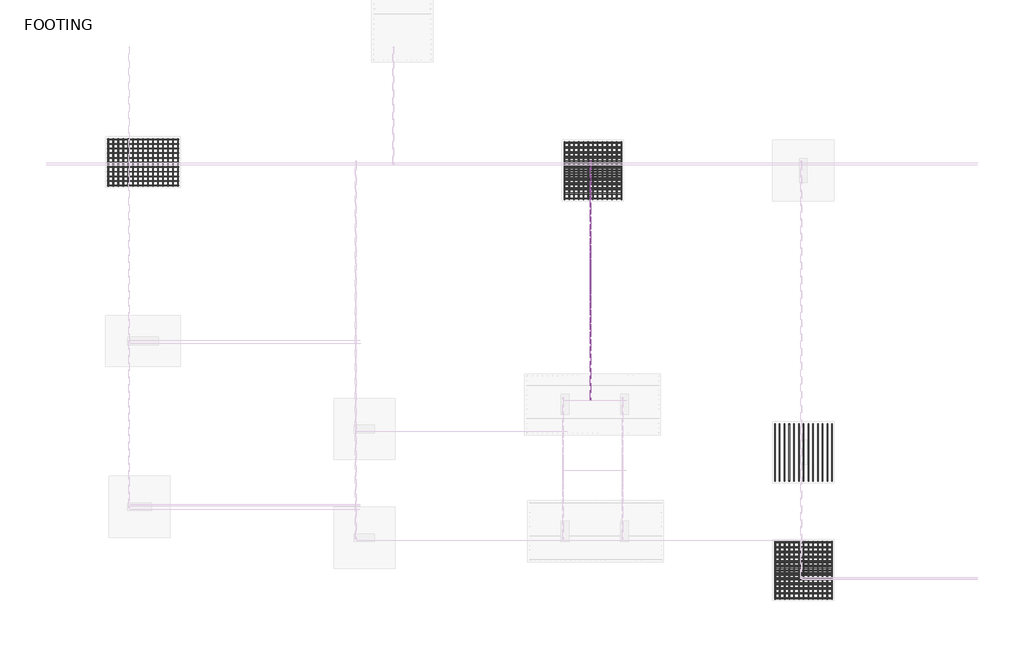
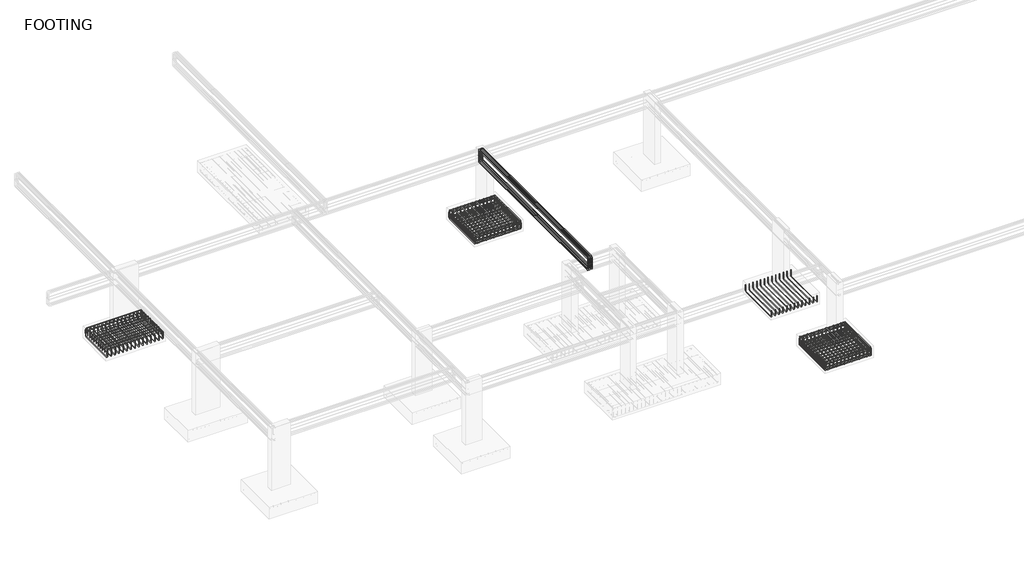
# One storey, part 5 of 12: 15 reinforcing bars.
"""IFC4 building model written with IfcOpenShell, lengths in millimetres."""

from ifc_helpers import new_model, si_unit, point, frame, origin, place, context, project, spatial, polyline, circle_curve, trimmed, segment, composite_curve, source, transform, mapped, element, save
from ifc_brep_helpers import swept_disk

model = new_model("IFC4")

# Units and contexts
model_context = context("Model", 3, world=origin())
ifc_project = project(units=[si_unit("LENGTHUNIT", "METRE", prefix="MILLI")], contexts=[model_context])

# Site, building, storey
site = spatial("IfcSite", under=ifc_project)
building = spatial("IfcBuilding", under=site)
storey = spatial("IfcBuildingStorey", under=building, Name="FOOTING", Elevation=-5638.8)

# Reinforcing bars
placement = place(None, origin())
reinforcing_bar_shape = source(origin(), model_context, "Body", "SolidModel", [
    swept_disk(composite_curve([segment(polyline([(5332.7998335, -15010.4541655, -5788.8), (5332.7998335, -15010.4541655, -5975.4)]), True, "CONTINUOUS"), segment(trimmed(circle_curve(frame((5332.7998335, -14955.0041655, -5975.4), z_axis=(1.0, 0.0, 0.0), x_axis=(0.0, -55.44999999999891, 0.0)), 55.45), [point((5332.7998335, -15010.4541655, -5975.4))], [point((5332.7998335, -14955.0041655, -6030.85))], True, "CARTESIAN"), True, "CONTINUOUS"), segment(polyline([(5332.7998335, -14955.0041655, -6030.85), (5332.7998335, -13381.8041655, -6030.85)]), True, "CONTINUOUS"), segment(trimmed(circle_curve(frame((5332.7998335, -13381.8041655, -5975.4), z_axis=(1.0, 0.0, 0.0), x_axis=(0.0, 0.0, -55.45000000000073)), 55.45), [point((5332.7998335, -13381.8041655, -6030.85))], [point((5332.7998335, -13326.3541655, -5975.4))], True, "CARTESIAN"), True, "CONTINUOUS"), segment(polyline([(5332.7998335, -13326.3541655, -5975.4), (5332.7998335, -13326.3541655, -5788.8)]), True, "CONTINUOUS")], self_intersect=False), 7.95),
])
element("IfcReinforcingBar", 1, at=placement, inside=storey, context=model_context, shape_type="MappedRepresentation", body=[
    mapped(reinforcing_bar_shape, transform((0.0, 0.0, 0.0), x_axis=(1.0, 0.0, 0.0), y_axis=(0.0, 1.0, 0.0), z_axis=(0.0, 0.0, 1.0))),
    mapped(reinforcing_bar_shape, transform((-140.3416667, 0.0, 0.0), x_axis=(1.0, 0.0, 0.0), y_axis=(0.0, 1.0, 0.0), z_axis=(0.0, 0.0, 1.0))),
    mapped(reinforcing_bar_shape, transform((-280.6833333, 0.0, 0.0), x_axis=(1.0, 0.0, 0.0), y_axis=(0.0, 1.0, 0.0), z_axis=(0.0, 0.0, 1.0))),
    mapped(reinforcing_bar_shape, transform((-421.025, 0.0, 0.0), x_axis=(1.0, 0.0, 0.0), y_axis=(0.0, 1.0, 0.0), z_axis=(0.0, 0.0, 1.0))),
    mapped(reinforcing_bar_shape, transform((-561.3666667, 0.0, 0.0), x_axis=(1.0, 0.0, 0.0), y_axis=(0.0, 1.0, 0.0), z_axis=(0.0, 0.0, 1.0))),
    mapped(reinforcing_bar_shape, transform((-701.7083333, 0.0, 0.0), x_axis=(1.0, 0.0, 0.0), y_axis=(0.0, 1.0, 0.0), z_axis=(0.0, 0.0, 1.0))),
    mapped(reinforcing_bar_shape, transform((-842.05, 0.0, 0.0), x_axis=(1.0, 0.0, 0.0), y_axis=(0.0, 1.0, 0.0), z_axis=(0.0, 0.0, 1.0))),
    mapped(reinforcing_bar_shape, transform((-982.3916667, 0.0, 0.0), x_axis=(1.0, 0.0, 0.0), y_axis=(0.0, 1.0, 0.0), z_axis=(0.0, 0.0, 1.0))),
    mapped(reinforcing_bar_shape, transform((-1122.7333333, 0.0, 0.0), x_axis=(1.0, 0.0, 0.0), y_axis=(0.0, 1.0, 0.0), z_axis=(0.0, 0.0, 1.0))),
    mapped(reinforcing_bar_shape, transform((-1263.075, 0.0, 0.0), x_axis=(1.0, 0.0, 0.0), y_axis=(0.0, 1.0, 0.0), z_axis=(0.0, 0.0, 1.0))),
    mapped(reinforcing_bar_shape, transform((-1403.4166667, 0.0, 0.0), x_axis=(1.0, 0.0, 0.0), y_axis=(0.0, 1.0, 0.0), z_axis=(0.0, 0.0, 1.0))),
    mapped(reinforcing_bar_shape, transform((-1543.7583333, 0.0, 0.0), x_axis=(1.0, 0.0, 0.0), y_axis=(0.0, 1.0, 0.0), z_axis=(0.0, 0.0, 1.0))),
    mapped(reinforcing_bar_shape, transform((-1684.1, 0.0, 0.0), x_axis=(1.0, 0.0, 0.0), y_axis=(0.0, 1.0, 0.0), z_axis=(0.0, 0.0, 1.0))),
])
reinforcing_bar_2_shape = source(origin(), model_context, "Body", "SolidModel", [
    swept_disk(composite_curve([segment(polyline([(5323.6597994, -13324.7541655, -5888.8), (5323.6597994, -13324.7541655, -5741.5)]), True, "CONTINUOUS"), segment(trimmed(circle_curve(frame((5323.6597994, -13371.1041655, -5741.5), z_axis=(1.0, 0.0, 0.0), x_axis=(0.0, 46.350000000000364, 0.0)), 46.35), [point((5323.6597994, -13324.7541655, -5741.5))], [point((5323.6597994, -13371.1041655, -5695.15))], True, "CARTESIAN"), True, "CONTINUOUS"), segment(polyline([(5323.6597994, -13371.1041655, -5695.15), (5323.6597994, -14965.7041655, -5695.15)]), True, "CONTINUOUS"), segment(trimmed(circle_curve(frame((5323.6597994, -14965.7041655, -5741.5), z_axis=(1.0, 0.0, 0.0), x_axis=(0.0, 0.0, 46.350000000000364)), 46.35), [point((5323.6597994, -14965.7041655, -5695.15))], [point((5323.6597994, -15012.0541655, -5741.5))], True, "CARTESIAN"), True, "CONTINUOUS"), segment(polyline([(5323.6597994, -15012.0541655, -5741.5), (5323.6597994, -15012.0541655, -5888.8)]), True, "CONTINUOUS")], self_intersect=False), 6.35),
])
element("IfcReinforcingBar", 2, at=placement, inside=storey, context=model_context, shape_type="MappedRepresentation", body=[
    mapped(reinforcing_bar_2_shape, transform((0.0, 0.0, 0.0), x_axis=(1.0, 0.0, 0.0), y_axis=(0.0, 1.0, 0.0), z_axis=(0.0, 0.0, 1.0))),
    mapped(reinforcing_bar_2_shape, transform((-138.4829293, 0.0, 0.0), x_axis=(1.0, 0.0, 0.0), y_axis=(0.0, 1.0, 0.0), z_axis=(0.0, 0.0, 1.0))),
    mapped(reinforcing_bar_2_shape, transform((-276.9658586, 0.0, 0.0), x_axis=(1.0, 0.0, 0.0), y_axis=(0.0, 1.0, 0.0), z_axis=(0.0, 0.0, 1.0))),
    mapped(reinforcing_bar_2_shape, transform((-415.4487879, 0.0, 0.0), x_axis=(1.0, 0.0, 0.0), y_axis=(0.0, 1.0, 0.0), z_axis=(0.0, 0.0, 1.0))),
    mapped(reinforcing_bar_2_shape, transform((-553.9317172, 0.0, 0.0), x_axis=(1.0, 0.0, 0.0), y_axis=(0.0, 1.0, 0.0), z_axis=(0.0, 0.0, 1.0))),
    mapped(reinforcing_bar_2_shape, transform((-692.4146465, 0.0, 0.0), x_axis=(1.0, 0.0, 0.0), y_axis=(0.0, 1.0, 0.0), z_axis=(0.0, 0.0, 1.0))),
    mapped(reinforcing_bar_2_shape, transform((-830.8975758, 0.0, 0.0), x_axis=(1.0, 0.0, 0.0), y_axis=(0.0, 1.0, 0.0), z_axis=(0.0, 0.0, 1.0))),
    mapped(reinforcing_bar_2_shape, transform((-969.3805051, 0.0, 0.0), x_axis=(1.0, 0.0, 0.0), y_axis=(0.0, 1.0, 0.0), z_axis=(0.0, 0.0, 1.0))),
    mapped(reinforcing_bar_2_shape, transform((-1107.8634344, 0.0, 0.0), x_axis=(1.0, 0.0, 0.0), y_axis=(0.0, 1.0, 0.0), z_axis=(0.0, 0.0, 1.0))),
    mapped(reinforcing_bar_2_shape, transform((-1246.3463637, 0.0, 0.0), x_axis=(1.0, 0.0, 0.0), y_axis=(0.0, 1.0, 0.0), z_axis=(0.0, 0.0, 1.0))),
    mapped(reinforcing_bar_2_shape, transform((-1384.8292929, 0.0, 0.0), x_axis=(1.0, 0.0, 0.0), y_axis=(0.0, 1.0, 0.0), z_axis=(0.0, 0.0, 1.0))),
    mapped(reinforcing_bar_2_shape, transform((-1523.3122222, 0.0, 0.0), x_axis=(1.0, 0.0, 0.0), y_axis=(0.0, 1.0, 0.0), z_axis=(0.0, 0.0, 1.0))),
    mapped(reinforcing_bar_2_shape, transform((-1661.7951515, 0.0, 0.0), x_axis=(1.0, 0.0, 0.0), y_axis=(0.0, 1.0, 0.0), z_axis=(0.0, 0.0, 1.0))),
])
reinforcing_bar_3_shape = source(origin(), model_context, "Body", "SolidModel", [
    swept_disk(composite_curve([segment(polyline([(3648.6998335, -14993.4041655, -5773.0), (3648.6998335, -14993.4041655, -5959.6)]), True, "CONTINUOUS"), segment(trimmed(circle_curve(frame((3704.1498335, -14993.4041655, -5959.6), z_axis=(0.0, -1.0, 0.0), x_axis=(-55.45000000000027, 0.0, 0.0)), 55.45), [point((3648.6998335, -14993.4041655, -5959.6))], [point((3704.1498335, -14993.4041655, -6015.05))], True, "CARTESIAN"), True, "CONTINUOUS"), segment(polyline([(3704.1498335, -14993.4041655, -6015.05), (5277.3498335, -14993.4041655, -6015.05)]), True, "CONTINUOUS"), segment(trimmed(circle_curve(frame((5277.3498335, -14993.4041655, -5959.6), z_axis=(0.0, -1.0, 0.0), x_axis=(0.0, 0.0, -55.44999999999982)), 55.45), [point((5277.3498335, -14993.4041655, -6015.05))], [point((5332.7998335, -14993.4041655, -5959.6))], True, "CARTESIAN"), True, "CONTINUOUS"), segment(polyline([(5332.7998335, -14993.4041655, -5959.6), (5332.7998335, -14993.4041655, -5773.0)]), True, "CONTINUOUS")], self_intersect=False), 7.95),
])
element("IfcReinforcingBar", 3, at=placement, inside=storey, context=model_context, shape_type="MappedRepresentation", body=[
    mapped(reinforcing_bar_3_shape, transform((0.0, 0.0, 0.0), x_axis=(1.0, 0.0, 0.0), y_axis=(0.0, 1.0, 0.0), z_axis=(0.0, 0.0, 1.0))),
    mapped(reinforcing_bar_3_shape, transform((0.0, 137.7402087, 0.0), x_axis=(1.0, 0.0, 0.0), y_axis=(0.0, 1.0, 0.0), z_axis=(0.0, 0.0, 1.0))),
    mapped(reinforcing_bar_3_shape, transform((0.0, 275.4804175, 0.0), x_axis=(1.0, 0.0, 0.0), y_axis=(0.0, 1.0, 0.0), z_axis=(0.0, 0.0, 1.0))),
    mapped(reinforcing_bar_3_shape, transform((0.0, 413.2206262, 0.0), x_axis=(1.0, 0.0, 0.0), y_axis=(0.0, 1.0, 0.0), z_axis=(0.0, 0.0, 1.0))),
    mapped(reinforcing_bar_3_shape, transform((0.0, 550.960835, 0.0), x_axis=(1.0, 0.0, 0.0), y_axis=(0.0, 1.0, 0.0), z_axis=(0.0, 0.0, 1.0))),
    mapped(reinforcing_bar_3_shape, transform((0.0, 688.7010437, 0.0), x_axis=(1.0, 0.0, 0.0), y_axis=(0.0, 1.0, 0.0), z_axis=(0.0, 0.0, 1.0))),
    mapped(reinforcing_bar_3_shape, transform((0.0, 826.4412525, 0.0), x_axis=(1.0, 0.0, 0.0), y_axis=(0.0, 1.0, 0.0), z_axis=(0.0, 0.0, 1.0))),
    mapped(reinforcing_bar_3_shape, transform((0.0, 964.1814612, 0.0), x_axis=(1.0, 0.0, 0.0), y_axis=(0.0, 1.0, 0.0), z_axis=(0.0, 0.0, 1.0))),
    mapped(reinforcing_bar_3_shape, transform((0.0, 1101.92167, 0.0), x_axis=(1.0, 0.0, 0.0), y_axis=(0.0, 1.0, 0.0), z_axis=(0.0, 0.0, 1.0))),
    mapped(reinforcing_bar_3_shape, transform((0.0, 1239.6618787, 0.0), x_axis=(1.0, 0.0, 0.0), y_axis=(0.0, 1.0, 0.0), z_axis=(0.0, 0.0, 1.0))),
    mapped(reinforcing_bar_3_shape, transform((0.0, 1377.4020875, 0.0), x_axis=(1.0, 0.0, 0.0), y_axis=(0.0, 1.0, 0.0), z_axis=(0.0, 0.0, 1.0))),
    mapped(reinforcing_bar_3_shape, transform((0.0, 1515.1422962, 0.0), x_axis=(1.0, 0.0, 0.0), y_axis=(0.0, 1.0, 0.0), z_axis=(0.0, 0.0, 1.0))),
    mapped(reinforcing_bar_3_shape, transform((0.0, 1652.882505, 0.0), x_axis=(1.0, 0.0, 0.0), y_axis=(0.0, 1.0, 0.0), z_axis=(0.0, 0.0, 1.0))),
])
reinforcing_bar_4_shape = source(origin(), model_context, "Body", "SolidModel", [
    swept_disk(composite_curve([segment(polyline([(3648.6998335, -13350.7399866, -5950.85), (3648.6998335, -13350.7399866, -5764.25)]), True, "CONTINUOUS"), segment(trimmed(circle_curve(frame((3704.1498335, -13350.7399866, -5764.25), z_axis=(0.0, 1.0, 0.0), x_axis=(-55.45000000000027, 0.0, 0.0)), 55.45), [point((3648.6998335, -13350.7399866, -5764.25))], [point((3704.1498335, -13350.7399866, -5708.8))], True, "CARTESIAN"), True, "CONTINUOUS"), segment(polyline([(3704.1498335, -13350.7399866, -5708.8), (5277.3498335, -13350.7399866, -5708.8)]), True, "CONTINUOUS"), segment(trimmed(circle_curve(frame((5277.3498335, -13350.7399866, -5764.25), z_axis=(0.0, 1.0, 0.0), x_axis=(0.0, 0.0, 55.44999999999982)), 55.45), [point((5277.3498335, -13350.7399866, -5708.8))], [point((5332.7998335, -13350.7399866, -5764.25))], True, "CARTESIAN"), True, "CONTINUOUS"), segment(polyline([(5332.7998335, -13350.7399866, -5764.25), (5332.7998335, -13350.7399866, -5950.85)]), True, "CONTINUOUS")], self_intersect=False), 7.95),
])
element("IfcReinforcingBar", 4, at=placement, inside=storey, context=model_context, shape_type="MappedRepresentation", body=[
    mapped(reinforcing_bar_4_shape, transform((0.0, 0.0, 0.0), x_axis=(1.0, 0.0, 0.0), y_axis=(0.0, 1.0, 0.0), z_axis=(0.0, 0.0, 1.0))),
    mapped(reinforcing_bar_4_shape, transform((0.0, -148.1882348, 0.0), x_axis=(1.0, 0.0, 0.0), y_axis=(0.0, 1.0, 0.0), z_axis=(0.0, 0.0, 1.0))),
    mapped(reinforcing_bar_4_shape, transform((0.0, -296.3764695, 0.0), x_axis=(1.0, 0.0, 0.0), y_axis=(0.0, 1.0, 0.0), z_axis=(0.0, 0.0, 1.0))),
    mapped(reinforcing_bar_4_shape, transform((0.0, -444.5647043, 0.0), x_axis=(1.0, 0.0, 0.0), y_axis=(0.0, 1.0, 0.0), z_axis=(0.0, 0.0, 1.0))),
    mapped(reinforcing_bar_4_shape, transform((0.0, -592.7529391, 0.0), x_axis=(1.0, 0.0, 0.0), y_axis=(0.0, 1.0, 0.0), z_axis=(0.0, 0.0, 1.0))),
    mapped(reinforcing_bar_4_shape, transform((0.0, -740.9411738, 0.0), x_axis=(1.0, 0.0, 0.0), y_axis=(0.0, 1.0, 0.0), z_axis=(0.0, 0.0, 1.0))),
    mapped(reinforcing_bar_4_shape, transform((0.0, -889.1294086, 0.0), x_axis=(1.0, 0.0, 0.0), y_axis=(0.0, 1.0, 0.0), z_axis=(0.0, 0.0, 1.0))),
    mapped(reinforcing_bar_4_shape, transform((0.0, -1037.3176434, 0.0), x_axis=(1.0, 0.0, 0.0), y_axis=(0.0, 1.0, 0.0), z_axis=(0.0, 0.0, 1.0))),
    mapped(reinforcing_bar_4_shape, transform((0.0, -1185.5058782, 0.0), x_axis=(1.0, 0.0, 0.0), y_axis=(0.0, 1.0, 0.0), z_axis=(0.0, 0.0, 1.0))),
    mapped(reinforcing_bar_4_shape, transform((0.0, -1333.6941129, 0.0), x_axis=(1.0, 0.0, 0.0), y_axis=(0.0, 1.0, 0.0), z_axis=(0.0, 0.0, 1.0))),
    mapped(reinforcing_bar_4_shape, transform((0.0, -1481.8823477, 0.0), x_axis=(1.0, 0.0, 0.0), y_axis=(0.0, 1.0, 0.0), z_axis=(0.0, 0.0, 1.0))),
    mapped(reinforcing_bar_4_shape, transform((0.0, -1630.0705825, 0.0), x_axis=(1.0, 0.0, 0.0), y_axis=(0.0, 1.0, 0.0), z_axis=(0.0, 0.0, 1.0))),
])
reinforcing_bar_5_shape = source(origin(), model_context, "Body", "SolidModel", [
    swept_disk(composite_curve([segment(polyline([(5332.7998335, -11543.3541655, -5788.8), (5332.7998335, -11543.3541655, -5975.4)]), True, "CONTINUOUS"), segment(trimmed(circle_curve(frame((5332.7998335, -11487.9041655, -5975.4), z_axis=(1.0, 0.0, 0.0), x_axis=(0.0, -55.45000000000073, 0.0)), 55.45), [point((5332.7998335, -11543.3541655, -5975.4))], [point((5332.7998335, -11487.9041655, -6030.85))], True, "CARTESIAN"), True, "CONTINUOUS"), segment(polyline([(5332.7998335, -11487.9041655, -6030.85), (5332.7998335, -9914.7041655, -6030.85)]), True, "CONTINUOUS"), segment(trimmed(circle_curve(frame((5332.7998335, -9914.7041655, -5975.4), z_axis=(1.0, 0.0, 0.0), x_axis=(0.0, 0.0, -55.45000000000073)), 55.45), [point((5332.7998335, -9914.7041655, -6030.85))], [point((5332.7998335, -9859.2541655, -5975.4))], True, "CARTESIAN"), True, "CONTINUOUS"), segment(polyline([(5332.7998335, -9859.2541655, -5975.4), (5332.7998335, -9859.2541655, -5788.8)]), True, "CONTINUOUS")], self_intersect=False), 7.95),
])
element("IfcReinforcingBar", 5, at=placement, inside=storey, context=model_context, shape_type="MappedRepresentation", body=[
    mapped(reinforcing_bar_5_shape, transform((0.0, 0.0, 0.0), x_axis=(1.0, 0.0, 0.0), y_axis=(0.0, 1.0, 0.0), z_axis=(0.0, 0.0, 1.0))),
    mapped(reinforcing_bar_5_shape, transform((-140.3416667, 0.0, 0.0), x_axis=(1.0, 0.0, 0.0), y_axis=(0.0, 1.0, 0.0), z_axis=(0.0, 0.0, 1.0))),
    mapped(reinforcing_bar_5_shape, transform((-280.6833333, 0.0, 0.0), x_axis=(1.0, 0.0, 0.0), y_axis=(0.0, 1.0, 0.0), z_axis=(0.0, 0.0, 1.0))),
    mapped(reinforcing_bar_5_shape, transform((-421.025, 0.0, 0.0), x_axis=(1.0, 0.0, 0.0), y_axis=(0.0, 1.0, 0.0), z_axis=(0.0, 0.0, 1.0))),
    mapped(reinforcing_bar_5_shape, transform((-561.3666667, 0.0, 0.0), x_axis=(1.0, 0.0, 0.0), y_axis=(0.0, 1.0, 0.0), z_axis=(0.0, 0.0, 1.0))),
    mapped(reinforcing_bar_5_shape, transform((-701.7083333, 0.0, 0.0), x_axis=(1.0, 0.0, 0.0), y_axis=(0.0, 1.0, 0.0), z_axis=(0.0, 0.0, 1.0))),
    mapped(reinforcing_bar_5_shape, transform((-842.05, 0.0, 0.0), x_axis=(1.0, 0.0, 0.0), y_axis=(0.0, 1.0, 0.0), z_axis=(0.0, 0.0, 1.0))),
    mapped(reinforcing_bar_5_shape, transform((-982.3916667, 0.0, 0.0), x_axis=(1.0, 0.0, 0.0), y_axis=(0.0, 1.0, 0.0), z_axis=(0.0, 0.0, 1.0))),
    mapped(reinforcing_bar_5_shape, transform((-1122.7333333, 0.0, 0.0), x_axis=(1.0, 0.0, 0.0), y_axis=(0.0, 1.0, 0.0), z_axis=(0.0, 0.0, 1.0))),
    mapped(reinforcing_bar_5_shape, transform((-1263.075, 0.0, 0.0), x_axis=(1.0, 0.0, 0.0), y_axis=(0.0, 1.0, 0.0), z_axis=(0.0, 0.0, 1.0))),
    mapped(reinforcing_bar_5_shape, transform((-1403.4166667, 0.0, 0.0), x_axis=(1.0, 0.0, 0.0), y_axis=(0.0, 1.0, 0.0), z_axis=(0.0, 0.0, 1.0))),
    mapped(reinforcing_bar_5_shape, transform((-1543.7583333, 0.0, 0.0), x_axis=(1.0, 0.0, 0.0), y_axis=(0.0, 1.0, 0.0), z_axis=(0.0, 0.0, 1.0))),
    mapped(reinforcing_bar_5_shape, transform((-1684.1, 0.0, 0.0), x_axis=(1.0, 0.0, 0.0), y_axis=(0.0, 1.0, 0.0), z_axis=(0.0, 0.0, 1.0))),
])
reinforcing_bar_6_shape = source(origin(), model_context, "Body", "SolidModel", [
    swept_disk(composite_curve([segment(polyline([(-864.8001665, -3250.2541655, -5788.8), (-864.8001665, -3250.2541655, -5975.4)]), True, "CONTINUOUS"), segment(trimmed(circle_curve(frame((-864.8001665, -3194.8041655, -5975.4), z_axis=(1.0, 0.0, 0.0), x_axis=(0.0, -55.44999999999982, 0.0)), 55.45), [point((-864.8001665, -3250.2541655, -5975.4))], [point((-864.8001665, -3194.8041655, -6030.85))], True, "CARTESIAN"), True, "CONTINUOUS"), segment(polyline([(-864.8001665, -3194.8041655, -6030.85), (-864.8001665, -1621.6041655, -6030.85)]), True, "CONTINUOUS"), segment(trimmed(circle_curve(frame((-864.8001665, -1621.6041655, -5975.4), z_axis=(1.0, 0.0, 0.0), x_axis=(0.0, 0.0, -55.45000000000073)), 55.45), [point((-864.8001665, -1621.6041655, -6030.85))], [point((-864.8001665, -1566.1541655, -5975.4))], True, "CARTESIAN"), True, "CONTINUOUS"), segment(polyline([(-864.8001665, -1566.1541655, -5975.4), (-864.8001665, -1566.1541655, -5788.8)]), True, "CONTINUOUS")], self_intersect=False), 7.95),
])
element("IfcReinforcingBar", 6, at=placement, inside=storey, context=model_context, shape_type="MappedRepresentation", body=[
    mapped(reinforcing_bar_6_shape, transform((0.0, 0.0, 0.0), x_axis=(1.0, 0.0, 0.0), y_axis=(0.0, 1.0, 0.0), z_axis=(0.0, 0.0, 1.0))),
    mapped(reinforcing_bar_6_shape, transform((-140.3416667, 0.0, 0.0), x_axis=(1.0, 0.0, 0.0), y_axis=(0.0, 1.0, 0.0), z_axis=(0.0, 0.0, 1.0))),
    mapped(reinforcing_bar_6_shape, transform((-280.6833333, 0.0, 0.0), x_axis=(1.0, 0.0, 0.0), y_axis=(0.0, 1.0, 0.0), z_axis=(0.0, 0.0, 1.0))),
    mapped(reinforcing_bar_6_shape, transform((-421.025, 0.0, 0.0), x_axis=(1.0, 0.0, 0.0), y_axis=(0.0, 1.0, 0.0), z_axis=(0.0, 0.0, 1.0))),
    mapped(reinforcing_bar_6_shape, transform((-561.3666667, 0.0, 0.0), x_axis=(1.0, 0.0, 0.0), y_axis=(0.0, 1.0, 0.0), z_axis=(0.0, 0.0, 1.0))),
    mapped(reinforcing_bar_6_shape, transform((-701.7083333, 0.0, 0.0), x_axis=(1.0, 0.0, 0.0), y_axis=(0.0, 1.0, 0.0), z_axis=(0.0, 0.0, 1.0))),
    mapped(reinforcing_bar_6_shape, transform((-842.05, 0.0, 0.0), x_axis=(1.0, 0.0, 0.0), y_axis=(0.0, 1.0, 0.0), z_axis=(0.0, 0.0, 1.0))),
    mapped(reinforcing_bar_6_shape, transform((-982.3916667, 0.0, 0.0), x_axis=(1.0, 0.0, 0.0), y_axis=(0.0, 1.0, 0.0), z_axis=(0.0, 0.0, 1.0))),
    mapped(reinforcing_bar_6_shape, transform((-1122.7333333, 0.0, 0.0), x_axis=(1.0, 0.0, 0.0), y_axis=(0.0, 1.0, 0.0), z_axis=(0.0, 0.0, 1.0))),
    mapped(reinforcing_bar_6_shape, transform((-1263.075, 0.0, 0.0), x_axis=(1.0, 0.0, 0.0), y_axis=(0.0, 1.0, 0.0), z_axis=(0.0, 0.0, 1.0))),
    mapped(reinforcing_bar_6_shape, transform((-1403.4166667, 0.0, 0.0), x_axis=(1.0, 0.0, 0.0), y_axis=(0.0, 1.0, 0.0), z_axis=(0.0, 0.0, 1.0))),
    mapped(reinforcing_bar_6_shape, transform((-1543.7583333, 0.0, 0.0), x_axis=(1.0, 0.0, 0.0), y_axis=(0.0, 1.0, 0.0), z_axis=(0.0, 0.0, 1.0))),
    mapped(reinforcing_bar_6_shape, transform((-1684.1, 0.0, 0.0), x_axis=(1.0, 0.0, 0.0), y_axis=(0.0, 1.0, 0.0), z_axis=(0.0, 0.0, 1.0))),
])
reinforcing_bar_7_shape = source(origin(), model_context, "Body", "SolidModel", [
    swept_disk(composite_curve([segment(polyline([(-873.9402006, -1564.5541655, -5888.8), (-873.9402006, -1564.5541655, -5741.5)]), True, "CONTINUOUS"), segment(trimmed(circle_curve(frame((-873.9402006, -1610.9041655, -5741.5), z_axis=(1.0, 0.0, 0.0), x_axis=(0.0, 46.350000000000136, 0.0)), 46.35), [point((-873.9402006, -1564.5541655, -5741.5))], [point((-873.9402006, -1610.9041655, -5695.15))], True, "CARTESIAN"), True, "CONTINUOUS"), segment(polyline([(-873.9402006, -1610.9041655, -5695.15), (-873.9402006, -3205.5041655, -5695.15)]), True, "CONTINUOUS"), segment(trimmed(circle_curve(frame((-873.9402006, -3205.5041655, -5741.5), z_axis=(1.0, 0.0, 0.0), x_axis=(0.0, 0.0, 46.350000000000364)), 46.35), [point((-873.9402006, -3205.5041655, -5695.15))], [point((-873.9402006, -3251.8541655, -5741.5))], True, "CARTESIAN"), True, "CONTINUOUS"), segment(polyline([(-873.9402006, -3251.8541655, -5741.5), (-873.9402006, -3251.8541655, -5888.8)]), True, "CONTINUOUS")], self_intersect=False), 6.35),
])
element("IfcReinforcingBar", 7, at=placement, inside=storey, context=model_context, shape_type="MappedRepresentation", body=[
    mapped(reinforcing_bar_7_shape, transform((0.0, 0.0, 0.0), x_axis=(1.0, 0.0, 0.0), y_axis=(0.0, 1.0, 0.0), z_axis=(0.0, 0.0, 1.0))),
    mapped(reinforcing_bar_7_shape, transform((-138.4829293, 0.0, 0.0), x_axis=(1.0, 0.0, 0.0), y_axis=(0.0, 1.0, 0.0), z_axis=(0.0, 0.0, 1.0))),
    mapped(reinforcing_bar_7_shape, transform((-276.9658586, 0.0, 0.0), x_axis=(1.0, 0.0, 0.0), y_axis=(0.0, 1.0, 0.0), z_axis=(0.0, 0.0, 1.0))),
    mapped(reinforcing_bar_7_shape, transform((-415.4487879, 0.0, 0.0), x_axis=(1.0, 0.0, 0.0), y_axis=(0.0, 1.0, 0.0), z_axis=(0.0, 0.0, 1.0))),
    mapped(reinforcing_bar_7_shape, transform((-553.9317172, 0.0, 0.0), x_axis=(1.0, 0.0, 0.0), y_axis=(0.0, 1.0, 0.0), z_axis=(0.0, 0.0, 1.0))),
    mapped(reinforcing_bar_7_shape, transform((-692.4146465, 0.0, 0.0), x_axis=(1.0, 0.0, 0.0), y_axis=(0.0, 1.0, 0.0), z_axis=(0.0, 0.0, 1.0))),
    mapped(reinforcing_bar_7_shape, transform((-830.8975758, 0.0, 0.0), x_axis=(1.0, 0.0, 0.0), y_axis=(0.0, 1.0, 0.0), z_axis=(0.0, 0.0, 1.0))),
    mapped(reinforcing_bar_7_shape, transform((-969.3805051, 0.0, 0.0), x_axis=(1.0, 0.0, 0.0), y_axis=(0.0, 1.0, 0.0), z_axis=(0.0, 0.0, 1.0))),
    mapped(reinforcing_bar_7_shape, transform((-1107.8634344, 0.0, 0.0), x_axis=(1.0, 0.0, 0.0), y_axis=(0.0, 1.0, 0.0), z_axis=(0.0, 0.0, 1.0))),
    mapped(reinforcing_bar_7_shape, transform((-1246.3463637, 0.0, 0.0), x_axis=(1.0, 0.0, 0.0), y_axis=(0.0, 1.0, 0.0), z_axis=(0.0, 0.0, 1.0))),
    mapped(reinforcing_bar_7_shape, transform((-1384.8292929, 0.0, 0.0), x_axis=(1.0, 0.0, 0.0), y_axis=(0.0, 1.0, 0.0), z_axis=(0.0, 0.0, 1.0))),
    mapped(reinforcing_bar_7_shape, transform((-1523.3122222, 0.0, 0.0), x_axis=(1.0, 0.0, 0.0), y_axis=(0.0, 1.0, 0.0), z_axis=(0.0, 0.0, 1.0))),
    mapped(reinforcing_bar_7_shape, transform((-1661.7951515, 0.0, 0.0), x_axis=(1.0, 0.0, 0.0), y_axis=(0.0, 1.0, 0.0), z_axis=(0.0, 0.0, 1.0))),
])
reinforcing_bar_8_shape = source(origin(), model_context, "Body", "SolidModel", [
    swept_disk(composite_curve([segment(polyline([(-2548.9001665, -3233.2041655, -5773.0), (-2548.9001665, -3233.2041655, -5959.6)]), True, "CONTINUOUS"), segment(trimmed(circle_curve(frame((-2493.4501665, -3233.2041655, -5959.6), z_axis=(0.0, -1.0, 0.0), x_axis=(-55.45000000000027, 0.0, 0.0)), 55.45), [point((-2548.9001665, -3233.2041655, -5959.6))], [point((-2493.4501665, -3233.2041655, -6015.05))], True, "CARTESIAN"), True, "CONTINUOUS"), segment(polyline([(-2493.4501665, -3233.2041655, -6015.05), (-920.2501665, -3233.2041655, -6015.05)]), True, "CONTINUOUS"), segment(trimmed(circle_curve(frame((-920.2501665, -3233.2041655, -5959.6), z_axis=(0.0, -1.0, 0.0), x_axis=(0.0, 0.0, -55.44999999999982)), 55.45), [point((-920.2501665, -3233.2041655, -6015.05))], [point((-864.8001665, -3233.2041655, -5959.6))], True, "CARTESIAN"), True, "CONTINUOUS"), segment(polyline([(-864.8001665, -3233.2041655, -5959.6), (-864.8001665, -3233.2041655, -5773.0)]), True, "CONTINUOUS")], self_intersect=False), 7.95),
])
element("IfcReinforcingBar", 8, at=placement, inside=storey, context=model_context, shape_type="MappedRepresentation", body=[
    mapped(reinforcing_bar_8_shape, transform((0.0, 0.0, 0.0), x_axis=(1.0, 0.0, 0.0), y_axis=(0.0, 1.0, 0.0), z_axis=(0.0, 0.0, 1.0))),
    mapped(reinforcing_bar_8_shape, transform((0.0, 137.7402087, 0.0), x_axis=(1.0, 0.0, 0.0), y_axis=(0.0, 1.0, 0.0), z_axis=(0.0, 0.0, 1.0))),
    mapped(reinforcing_bar_8_shape, transform((0.0, 275.4804175, 0.0), x_axis=(1.0, 0.0, 0.0), y_axis=(0.0, 1.0, 0.0), z_axis=(0.0, 0.0, 1.0))),
    mapped(reinforcing_bar_8_shape, transform((0.0, 413.2206262, 0.0), x_axis=(1.0, 0.0, 0.0), y_axis=(0.0, 1.0, 0.0), z_axis=(0.0, 0.0, 1.0))),
    mapped(reinforcing_bar_8_shape, transform((0.0, 550.960835, 0.0), x_axis=(1.0, 0.0, 0.0), y_axis=(0.0, 1.0, 0.0), z_axis=(0.0, 0.0, 1.0))),
    mapped(reinforcing_bar_8_shape, transform((0.0, 688.7010437, 0.0), x_axis=(1.0, 0.0, 0.0), y_axis=(0.0, 1.0, 0.0), z_axis=(0.0, 0.0, 1.0))),
    mapped(reinforcing_bar_8_shape, transform((0.0, 826.4412525, 0.0), x_axis=(1.0, 0.0, 0.0), y_axis=(0.0, 1.0, 0.0), z_axis=(0.0, 0.0, 1.0))),
    mapped(reinforcing_bar_8_shape, transform((0.0, 964.1814612, 0.0), x_axis=(1.0, 0.0, 0.0), y_axis=(0.0, 1.0, 0.0), z_axis=(0.0, 0.0, 1.0))),
    mapped(reinforcing_bar_8_shape, transform((0.0, 1101.92167, 0.0), x_axis=(1.0, 0.0, 0.0), y_axis=(0.0, 1.0, 0.0), z_axis=(0.0, 0.0, 1.0))),
    mapped(reinforcing_bar_8_shape, transform((0.0, 1239.6618787, 0.0), x_axis=(1.0, 0.0, 0.0), y_axis=(0.0, 1.0, 0.0), z_axis=(0.0, 0.0, 1.0))),
    mapped(reinforcing_bar_8_shape, transform((0.0, 1377.4020875, 0.0), x_axis=(1.0, 0.0, 0.0), y_axis=(0.0, 1.0, 0.0), z_axis=(0.0, 0.0, 1.0))),
    mapped(reinforcing_bar_8_shape, transform((0.0, 1515.1422962, 0.0), x_axis=(1.0, 0.0, 0.0), y_axis=(0.0, 1.0, 0.0), z_axis=(0.0, 0.0, 1.0))),
    mapped(reinforcing_bar_8_shape, transform((0.0, 1652.882505, 0.0), x_axis=(1.0, 0.0, 0.0), y_axis=(0.0, 1.0, 0.0), z_axis=(0.0, 0.0, 1.0))),
])
reinforcing_bar_9_shape = source(origin(), model_context, "Body", "SolidModel", [
    swept_disk(composite_curve([segment(polyline([(-2548.9001665, -1590.5399866, -5950.85), (-2548.9001665, -1590.5399866, -5764.25)]), True, "CONTINUOUS"), segment(trimmed(circle_curve(frame((-2493.4501665, -1590.5399866, -5764.25), z_axis=(0.0, 1.0, 0.0), x_axis=(-55.45000000000027, 0.0, 0.0)), 55.45), [point((-2548.9001665, -1590.5399866, -5764.25))], [point((-2493.4501665, -1590.5399866, -5708.8))], True, "CARTESIAN"), True, "CONTINUOUS"), segment(polyline([(-2493.4501665, -1590.5399866, -5708.8), (-920.2501665, -1590.5399866, -5708.8)]), True, "CONTINUOUS"), segment(trimmed(circle_curve(frame((-920.2501665, -1590.5399866, -5764.25), z_axis=(0.0, 1.0, 0.0), x_axis=(0.0, 0.0, 55.44999999999982)), 55.45), [point((-920.2501665, -1590.5399866, -5708.8))], [point((-864.8001665, -1590.5399866, -5764.25))], True, "CARTESIAN"), True, "CONTINUOUS"), segment(polyline([(-864.8001665, -1590.5399866, -5764.25), (-864.8001665, -1590.5399866, -5950.85)]), True, "CONTINUOUS")], self_intersect=False), 7.95),
])
element("IfcReinforcingBar", 9, at=placement, inside=storey, context=model_context, shape_type="MappedRepresentation", body=[
    mapped(reinforcing_bar_9_shape, transform((0.0, 0.0, 0.0), x_axis=(1.0, 0.0, 0.0), y_axis=(0.0, 1.0, 0.0), z_axis=(0.0, 0.0, 1.0))),
    mapped(reinforcing_bar_9_shape, transform((0.0, -148.1882348, 0.0), x_axis=(1.0, 0.0, 0.0), y_axis=(0.0, 1.0, 0.0), z_axis=(0.0, 0.0, 1.0))),
    mapped(reinforcing_bar_9_shape, transform((0.0, -296.3764695, 0.0), x_axis=(1.0, 0.0, 0.0), y_axis=(0.0, 1.0, 0.0), z_axis=(0.0, 0.0, 1.0))),
    mapped(reinforcing_bar_9_shape, transform((0.0, -444.5647043, 0.0), x_axis=(1.0, 0.0, 0.0), y_axis=(0.0, 1.0, 0.0), z_axis=(0.0, 0.0, 1.0))),
    mapped(reinforcing_bar_9_shape, transform((0.0, -592.7529391, 0.0), x_axis=(1.0, 0.0, 0.0), y_axis=(0.0, 1.0, 0.0), z_axis=(0.0, 0.0, 1.0))),
    mapped(reinforcing_bar_9_shape, transform((0.0, -740.9411738, 0.0), x_axis=(1.0, 0.0, 0.0), y_axis=(0.0, 1.0, 0.0), z_axis=(0.0, 0.0, 1.0))),
    mapped(reinforcing_bar_9_shape, transform((0.0, -889.1294086, 0.0), x_axis=(1.0, 0.0, 0.0), y_axis=(0.0, 1.0, 0.0), z_axis=(0.0, 0.0, 1.0))),
    mapped(reinforcing_bar_9_shape, transform((0.0, -1037.3176434, 0.0), x_axis=(1.0, 0.0, 0.0), y_axis=(0.0, 1.0, 0.0), z_axis=(0.0, 0.0, 1.0))),
    mapped(reinforcing_bar_9_shape, transform((0.0, -1185.5058782, 0.0), x_axis=(1.0, 0.0, 0.0), y_axis=(0.0, 1.0, 0.0), z_axis=(0.0, 0.0, 1.0))),
    mapped(reinforcing_bar_9_shape, transform((0.0, -1333.6941129, 0.0), x_axis=(1.0, 0.0, 0.0), y_axis=(0.0, 1.0, 0.0), z_axis=(0.0, 0.0, 1.0))),
    mapped(reinforcing_bar_9_shape, transform((0.0, -1481.8823477, 0.0), x_axis=(1.0, 0.0, 0.0), y_axis=(0.0, 1.0, 0.0), z_axis=(0.0, 0.0, 1.0))),
    mapped(reinforcing_bar_9_shape, transform((0.0, -1630.0705825, 0.0), x_axis=(1.0, 0.0, 0.0), y_axis=(0.0, 1.0, 0.0), z_axis=(0.0, 0.0, 1.0))),
])
reinforcing_bar_10_shape = source(origin(), model_context, "Body", "SolidModel", [
    swept_disk(composite_curve([segment(polyline([(-13896.6001665, -2847.7545193, -5888.8), (-13896.6001665, -2847.7545193, -5741.5)]), True, "CONTINUOUS"), segment(trimmed(circle_curve(frame((-13942.9501665, -2847.7545193, -5741.5), z_axis=(0.0, -1.0, 0.0), x_axis=(46.350000000000364, 0.0, 0.0)), 46.35), [point((-13896.6001665, -2847.7545193, -5741.5))], [point((-13942.9501665, -2847.7545193, -5695.15))], True, "CARTESIAN"), True, "CONTINUOUS"), segment(polyline([(-13942.9501665, -2847.7545193, -5695.15), (-15937.5501665, -2847.7545193, -5695.15)]), True, "CONTINUOUS"), segment(trimmed(circle_curve(frame((-15937.5501665, -2847.7545193, -5741.5), z_axis=(0.0, -1.0, 0.0), x_axis=(0.0, 0.0, 46.350000000000364)), 46.35), [point((-15937.5501665, -2847.7545193, -5695.15))], [point((-15983.9001665, -2847.7545193, -5741.5))], True, "CARTESIAN"), True, "CONTINUOUS"), segment(polyline([(-15983.9001665, -2847.7545193, -5741.5), (-15983.9001665, -2847.7545193, -5888.8)]), True, "CONTINUOUS")], self_intersect=False), 6.35),
])
element("IfcReinforcingBar", 10, at=placement, inside=storey, context=model_context, shape_type="MappedRepresentation", body=[
    mapped(reinforcing_bar_10_shape, transform((0.0, 0.0, 0.0), x_axis=(1.0, 0.0, 0.0), y_axis=(0.0, 1.0, 0.0), z_axis=(0.0, 0.0, 1.0))),
    mapped(reinforcing_bar_10_shape, transform((0.0, 136.1586067, 0.0), x_axis=(1.0, 0.0, 0.0), y_axis=(0.0, 1.0, 0.0), z_axis=(0.0, 0.0, 1.0))),
    mapped(reinforcing_bar_10_shape, transform((0.0, 272.3172133, 0.0), x_axis=(1.0, 0.0, 0.0), y_axis=(0.0, 1.0, 0.0), z_axis=(0.0, 0.0, 1.0))),
    mapped(reinforcing_bar_10_shape, transform((0.0, 408.47582, 0.0), x_axis=(1.0, 0.0, 0.0), y_axis=(0.0, 1.0, 0.0), z_axis=(0.0, 0.0, 1.0))),
    mapped(reinforcing_bar_10_shape, transform((0.0, 544.6344267, 0.0), x_axis=(1.0, 0.0, 0.0), y_axis=(0.0, 1.0, 0.0), z_axis=(0.0, 0.0, 1.0))),
    mapped(reinforcing_bar_10_shape, transform((0.0, 680.7930333, 0.0), x_axis=(1.0, 0.0, 0.0), y_axis=(0.0, 1.0, 0.0), z_axis=(0.0, 0.0, 1.0))),
    mapped(reinforcing_bar_10_shape, transform((0.0, 816.95164, 0.0), x_axis=(1.0, 0.0, 0.0), y_axis=(0.0, 1.0, 0.0), z_axis=(0.0, 0.0, 1.0))),
    mapped(reinforcing_bar_10_shape, transform((0.0, 953.1102467, 0.0), x_axis=(1.0, 0.0, 0.0), y_axis=(0.0, 1.0, 0.0), z_axis=(0.0, 0.0, 1.0))),
    mapped(reinforcing_bar_10_shape, transform((0.0, 1089.2688533, 0.0), x_axis=(1.0, 0.0, 0.0), y_axis=(0.0, 1.0, 0.0), z_axis=(0.0, 0.0, 1.0))),
    mapped(reinforcing_bar_10_shape, transform((0.0, 1225.42746, 0.0), x_axis=(1.0, 0.0, 0.0), y_axis=(0.0, 1.0, 0.0), z_axis=(0.0, 0.0, 1.0))),
    mapped(reinforcing_bar_10_shape, transform((0.0, 1361.5860667, 0.0), x_axis=(1.0, 0.0, 0.0), y_axis=(0.0, 1.0, 0.0), z_axis=(0.0, 0.0, 1.0))),
])
reinforcing_bar_11_shape = source(origin(), model_context, "Body", "SolidModel", [
    swept_disk(composite_curve([segment(polyline([(-15971.9866414, -1473.2541655, -5821.490176), (-15971.9866414, -1473.2541655, -5968.790176)]), True, "CONTINUOUS"), segment(trimmed(circle_curve(frame((-15971.9866414, -1519.6041655, -5968.790176), z_axis=(-1.0, 0.0, 0.0), x_axis=(0.0, 46.34999999999991, 0.0)), 46.35), [point((-15971.9866414, -1473.2541655, -5968.790176))], [point((-15971.9866414, -1519.6041655, -6015.140176))], True, "CARTESIAN"), True, "CONTINUOUS"), segment(polyline([(-15971.9866414, -1519.6041655, -6015.140176), (-15971.9866414, -2814.2041655, -6015.140176)]), True, "CONTINUOUS"), segment(trimmed(circle_curve(frame((-15971.9866414, -2814.2041655, -5968.790176), z_axis=(-1.0, 0.0, 0.0), x_axis=(0.0, 0.0, -46.349999999999454)), 46.35), [point((-15971.9866414, -2814.2041655, -6015.140176))], [point((-15971.9866414, -2860.5541655, -5968.790176))], True, "CARTESIAN"), True, "CONTINUOUS"), segment(polyline([(-15971.9866414, -2860.5541655, -5968.790176), (-15971.9866414, -2860.5541655, -5821.490176)]), True, "CONTINUOUS")], self_intersect=False), 6.35),
])
element("IfcReinforcingBar", 11, at=placement, inside=storey, context=model_context, shape_type="MappedRepresentation", body=[
    mapped(reinforcing_bar_11_shape, transform((0.0, 0.0, 0.0), x_axis=(1.0, 0.0, 0.0), y_axis=(0.0, 1.0, 0.0), z_axis=(0.0, 0.0, 1.0))),
    mapped(reinforcing_bar_11_shape, transform((147.43641, 0.0, 0.0), x_axis=(1.0, 0.0, 0.0), y_axis=(0.0, 1.0, 0.0), z_axis=(0.0, 0.0, 1.0))),
    mapped(reinforcing_bar_11_shape, transform((294.87282, 0.0, 0.0), x_axis=(1.0, 0.0, 0.0), y_axis=(0.0, 1.0, 0.0), z_axis=(0.0, 0.0, 1.0))),
    mapped(reinforcing_bar_11_shape, transform((442.30923, 0.0, 0.0), x_axis=(1.0, 0.0, 0.0), y_axis=(0.0, 1.0, 0.0), z_axis=(0.0, 0.0, 1.0))),
    mapped(reinforcing_bar_11_shape, transform((589.74564, 0.0, 0.0), x_axis=(1.0, 0.0, 0.0), y_axis=(0.0, 1.0, 0.0), z_axis=(0.0, 0.0, 1.0))),
    mapped(reinforcing_bar_11_shape, transform((737.1820499, 0.0, 0.0), x_axis=(1.0, 0.0, 0.0), y_axis=(0.0, 1.0, 0.0), z_axis=(0.0, 0.0, 1.0))),
    mapped(reinforcing_bar_11_shape, transform((884.6184599, 0.0, 0.0), x_axis=(1.0, 0.0, 0.0), y_axis=(0.0, 1.0, 0.0), z_axis=(0.0, 0.0, 1.0))),
    mapped(reinforcing_bar_11_shape, transform((1032.0548699, 0.0, 0.0), x_axis=(1.0, 0.0, 0.0), y_axis=(0.0, 1.0, 0.0), z_axis=(0.0, 0.0, 1.0))),
    mapped(reinforcing_bar_11_shape, transform((1179.4912799, 0.0, 0.0), x_axis=(1.0, 0.0, 0.0), y_axis=(0.0, 1.0, 0.0), z_axis=(0.0, 0.0, 1.0))),
    mapped(reinforcing_bar_11_shape, transform((1326.9276899, 0.0, 0.0), x_axis=(1.0, 0.0, 0.0), y_axis=(0.0, 1.0, 0.0), z_axis=(0.0, 0.0, 1.0))),
    mapped(reinforcing_bar_11_shape, transform((1474.3640999, 0.0, 0.0), x_axis=(1.0, 0.0, 0.0), y_axis=(0.0, 1.0, 0.0), z_axis=(0.0, 0.0, 1.0))),
    mapped(reinforcing_bar_11_shape, transform((1621.8005099, 0.0, 0.0), x_axis=(1.0, 0.0, 0.0), y_axis=(0.0, 1.0, 0.0), z_axis=(0.0, 0.0, 1.0))),
    mapped(reinforcing_bar_11_shape, transform((1769.2369199, 0.0, 0.0), x_axis=(1.0, 0.0, 0.0), y_axis=(0.0, 1.0, 0.0), z_axis=(0.0, 0.0, 1.0))),
    mapped(reinforcing_bar_11_shape, transform((1916.6733299, 0.0, 0.0), x_axis=(1.0, 0.0, 0.0), y_axis=(0.0, 1.0, 0.0), z_axis=(0.0, 0.0, 1.0))),
    mapped(reinforcing_bar_11_shape, transform((2064.1097398, 0.0, 0.0), x_axis=(1.0, 0.0, 0.0), y_axis=(0.0, 1.0, 0.0), z_axis=(0.0, 0.0, 1.0))),
])
reinforcing_bar_12_shape = source(origin(), model_context, "Body", "SolidModel", [
    swept_disk(composite_curve([segment(polyline([(-13921.5742888, -1473.2541655, -5898.1017616), (-13921.5742888, -1473.2541655, -5750.8017616)]), True, "CONTINUOUS"), segment(trimmed(circle_curve(frame((-13921.5742888, -1519.6041655, -5750.8017616), z_axis=(1.0, 0.0, 0.0), x_axis=(0.0, 46.34999999999991, 0.0)), 46.35), [point((-13921.5742888, -1473.2541655, -5750.8017616))], [point((-13921.5742888, -1519.6041655, -5704.4517616))], True, "CARTESIAN"), True, "CONTINUOUS"), segment(polyline([(-13921.5742888, -1519.6041655, -5704.4517616), (-13921.5742888, -2814.2041655, -5704.4517616)]), True, "CONTINUOUS"), segment(trimmed(circle_curve(frame((-13921.5742888, -2814.2041655, -5750.8017616), z_axis=(1.0, 0.0, 0.0), x_axis=(0.0, 0.0, 46.349999999999454)), 46.35), [point((-13921.5742888, -2814.2041655, -5704.4517616))], [point((-13921.5742888, -2860.5541655, -5750.8017616))], True, "CARTESIAN"), True, "CONTINUOUS"), segment(polyline([(-13921.5742888, -2860.5541655, -5750.8017616), (-13921.5742888, -2860.5541655, -5898.1017616)]), True, "CONTINUOUS")], self_intersect=False), 6.35),
])
element("IfcReinforcingBar", 12, at=placement, inside=storey, context=model_context, shape_type="MappedRepresentation", body=[
    mapped(reinforcing_bar_12_shape, transform((0.0, 0.0, 0.0), x_axis=(1.0, 0.0, 0.0), y_axis=(0.0, 1.0, 0.0), z_axis=(0.0, 0.0, 1.0))),
    mapped(reinforcing_bar_12_shape, transform((-145.5195783, 0.0, 0.0), x_axis=(1.0, 0.0, 0.0), y_axis=(0.0, 1.0, 0.0), z_axis=(0.0, 0.0, 1.0))),
    mapped(reinforcing_bar_12_shape, transform((-291.0391566, 0.0, 0.0), x_axis=(1.0, 0.0, 0.0), y_axis=(0.0, 1.0, 0.0), z_axis=(0.0, 0.0, 1.0))),
    mapped(reinforcing_bar_12_shape, transform((-436.5587348, 0.0, 0.0), x_axis=(1.0, 0.0, 0.0), y_axis=(0.0, 1.0, 0.0), z_axis=(0.0, 0.0, 1.0))),
    mapped(reinforcing_bar_12_shape, transform((-582.0783131, 0.0, 0.0), x_axis=(1.0, 0.0, 0.0), y_axis=(0.0, 1.0, 0.0), z_axis=(0.0, 0.0, 1.0))),
    mapped(reinforcing_bar_12_shape, transform((-727.5978914, 0.0, 0.0), x_axis=(1.0, 0.0, 0.0), y_axis=(0.0, 1.0, 0.0), z_axis=(0.0, 0.0, 1.0))),
    mapped(reinforcing_bar_12_shape, transform((-873.1174697, 0.0, 0.0), x_axis=(1.0, 0.0, 0.0), y_axis=(0.0, 1.0, 0.0), z_axis=(0.0, 0.0, 1.0))),
    mapped(reinforcing_bar_12_shape, transform((-1018.637048, 0.0, 0.0), x_axis=(1.0, 0.0, 0.0), y_axis=(0.0, 1.0, 0.0), z_axis=(0.0, 0.0, 1.0))),
    mapped(reinforcing_bar_12_shape, transform((-1164.1566263, 0.0, 0.0), x_axis=(1.0, 0.0, 0.0), y_axis=(0.0, 1.0, 0.0), z_axis=(0.0, 0.0, 1.0))),
    mapped(reinforcing_bar_12_shape, transform((-1309.6762045, 0.0, 0.0), x_axis=(1.0, 0.0, 0.0), y_axis=(0.0, 1.0, 0.0), z_axis=(0.0, 0.0, 1.0))),
    mapped(reinforcing_bar_12_shape, transform((-1455.1957828, 0.0, 0.0), x_axis=(1.0, 0.0, 0.0), y_axis=(0.0, 1.0, 0.0), z_axis=(0.0, 0.0, 1.0))),
    mapped(reinforcing_bar_12_shape, transform((-1600.7153611, 0.0, 0.0), x_axis=(1.0, 0.0, 0.0), y_axis=(0.0, 1.0, 0.0), z_axis=(0.0, 0.0, 1.0))),
    mapped(reinforcing_bar_12_shape, transform((-1746.2349394, 0.0, 0.0), x_axis=(1.0, 0.0, 0.0), y_axis=(0.0, 1.0, 0.0), z_axis=(0.0, 0.0, 1.0))),
    mapped(reinforcing_bar_12_shape, transform((-1891.7545177, 0.0, 0.0), x_axis=(1.0, 0.0, 0.0), y_axis=(0.0, 1.0, 0.0), z_axis=(0.0, 0.0, 1.0))),
    mapped(reinforcing_bar_12_shape, transform((-2037.2740959, 0.0, 0.0), x_axis=(1.0, 0.0, 0.0), y_axis=(0.0, 1.0, 0.0), z_axis=(0.0, 0.0, 1.0))),
])
reinforcing_bar_13_shape = source(origin(), model_context, "Body", "SolidModel", [
    swept_disk(composite_curve([segment(polyline([(-1635.0001665, -9153.6326678, -3500.1457532), (-1635.0001665, -2115.7280815, -3500.1457532)]), True, "CONTINUOUS")], self_intersect=False), 7.95),
])
element("IfcReinforcingBar", 13, at=placement, inside=storey, context=model_context, shape_type="MappedRepresentation", body=[
    mapped(reinforcing_bar_13_shape, transform((0.0, 0.0, 0.0), x_axis=(1.0, 0.0, 0.0), y_axis=(0.0, 1.0, 0.0), z_axis=(0.0, 0.0, 1.0))),
    mapped(reinforcing_bar_13_shape, transform((-143.7, 0.0, 0.0), x_axis=(1.0, 0.0, 0.0), y_axis=(0.0, 1.0, 0.0), z_axis=(0.0, 0.0, 1.0))),
])
reinforcing_bar_14_shape = source(origin(), model_context, "Body", "SolidModel", [
    swept_disk(composite_curve([segment(polyline([(-1638.5295298, -9147.4323768, -3488.4293633), (-1638.5295298, -9147.4323768, -3301.8293633)]), True, "CONTINUOUS"), segment(trimmed(circle_curve(frame((-1638.5295298, -9091.9823768, -3301.8293633), z_axis=(-1.0, 0.0, 0.0), x_axis=(0.0, -55.44999999999891, 0.0)), 55.45), [point((-1638.5295298, -9147.4323768, -3301.8293633))], [point((-1638.5295298, -9091.9823768, -3246.3793633))], True, "CARTESIAN"), True, "CONTINUOUS"), segment(polyline([(-1638.5295298, -9091.9823768, -3246.3793633), (-1638.5295298, -2179.1027895, -3246.3793633)]), True, "CONTINUOUS"), segment(trimmed(circle_curve(frame((-1638.5295298, -2179.1027895, -3301.8293633), z_axis=(-1.0, 0.0, 0.0), x_axis=(0.0, 0.0, 55.44999999999982)), 55.45), [point((-1638.5295298, -2179.1027895, -3246.3793633))], [point((-1638.5295298, -2123.6527895, -3301.8293633))], True, "CARTESIAN"), True, "CONTINUOUS"), segment(polyline([(-1638.5295298, -2123.6527895, -3301.8293633), (-1638.5295298, -2123.6527895, -3488.4293633)]), True, "CONTINUOUS")], self_intersect=False), 7.95),
])
element("IfcReinforcingBar", 14, at=placement, inside=storey, context=model_context, shape_type="MappedRepresentation", body=[
    mapped(reinforcing_bar_14_shape, transform((0.0, 0.0, 0.0), x_axis=(1.0, 0.0, 0.0), y_axis=(0.0, 1.0, 0.0), z_axis=(0.0, 0.0, 1.0))),
    mapped(reinforcing_bar_14_shape, transform((-45.5470911, 0.0, 0.0), x_axis=(1.0, 0.0, 0.0), y_axis=(0.0, 1.0, 0.0), z_axis=(0.0, 0.0, 1.0))),
    mapped(reinforcing_bar_14_shape, transform((-91.0941823, 0.0, 0.0), x_axis=(1.0, 0.0, 0.0), y_axis=(0.0, 1.0, 0.0), z_axis=(0.0, 0.0, 1.0))),
    mapped(reinforcing_bar_14_shape, transform((-136.6412734, 0.0, 0.0), x_axis=(1.0, 0.0, 0.0), y_axis=(0.0, 1.0, 0.0), z_axis=(0.0, 0.0, 1.0))),
])
reinforcing_bar_15_shape = source(origin(), model_context, "Body", "SolidModel", [
    swept_disk(composite_curve([segment(polyline([(-1638.5295298, -9150.5871404, -3512.3706367), (-1638.5295298, -9150.5871404, -3698.9706367)]), True, "CONTINUOUS"), segment(trimmed(circle_curve(frame((-1638.5295298, -9095.1371404, -3698.9706367), z_axis=(1.0, 0.0, 0.0), x_axis=(0.0, -55.45000000000073, 0.0)), 55.45), [point((-1638.5295298, -9150.5871404, -3698.9706367))], [point((-1638.5295298, -9095.1371404, -3754.4206367))], True, "CARTESIAN"), True, "CONTINUOUS"), segment(polyline([(-1638.5295298, -9095.1371404, -3754.4206367), (-1638.5295298, -2183.4229247, -3754.4206367)]), True, "CONTINUOUS"), segment(trimmed(circle_curve(frame((-1638.5295298, -2183.4229247, -3698.9706367), z_axis=(1.0, 0.0, 0.0), x_axis=(0.0, 0.0, -55.45000000000027)), 55.45), [point((-1638.5295298, -2183.4229247, -3754.4206367))], [point((-1638.5295298, -2127.9729247, -3698.9706367))], True, "CARTESIAN"), True, "CONTINUOUS"), segment(polyline([(-1638.5295298, -2127.9729247, -3698.9706367), (-1638.5295298, -2127.9729247, -3512.3706367)]), True, "CONTINUOUS")], self_intersect=False), 7.95),
])
element("IfcReinforcingBar", 15, at=placement, inside=storey, context=model_context, shape_type="MappedRepresentation", body=[
    mapped(reinforcing_bar_15_shape, transform((0.0, 0.0, 0.0), x_axis=(1.0, 0.0, 0.0), y_axis=(0.0, 1.0, 0.0), z_axis=(0.0, 0.0, 1.0))),
    mapped(reinforcing_bar_15_shape, transform((-68.3206367, 0.0, 0.0), x_axis=(1.0, 0.0, 0.0), y_axis=(0.0, 1.0, 0.0), z_axis=(0.0, 0.0, 1.0))),
    mapped(reinforcing_bar_15_shape, transform((-136.6412734, 0.0, 0.0), x_axis=(1.0, 0.0, 0.0), y_axis=(0.0, 1.0, 0.0), z_axis=(0.0, 0.0, 1.0))),
])

save(model, "model.ifc")

# Revit data of these elements
# Elements 1, 2, 3, 4, 5, 6, 7, 8, 9, 10, 11, 12, 13, 14, 15 (IfcReinforcingBar)
#   Phase Created = New Construction
